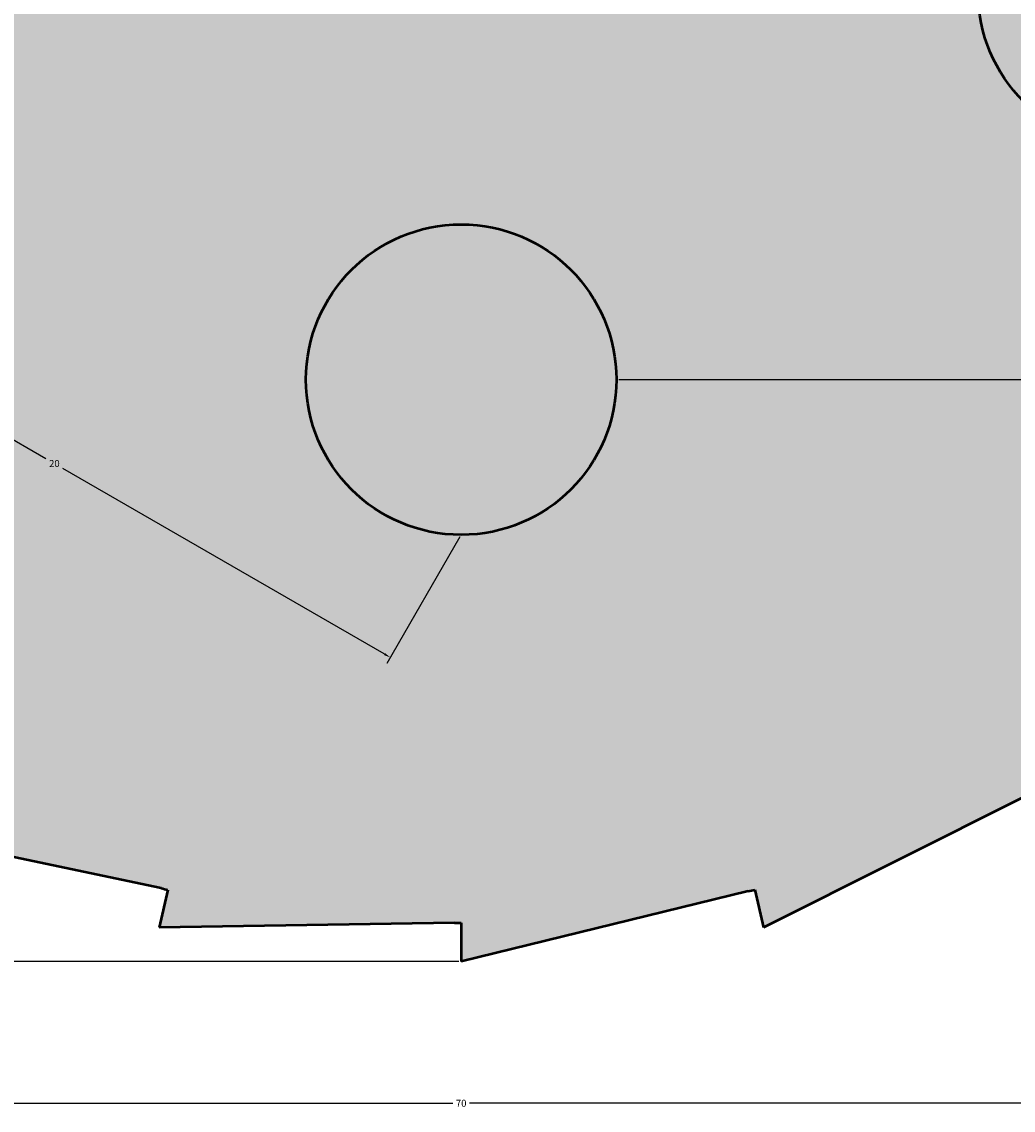
# Model space of a CAD drawing. Units: millimetres. Extents: x 2943.6 to 3032.7, y 1562 to 1639.7.
# Tile 2 of 9: x 2971.1 to 2996.7, y 1562 to 1590.1. Entities that reach past the tile are written whole.
import ezdxf

# ---------------------------------------------------------------- set-up
doc = ezdxf.new("R2010")
doc.units = ezdxf.units.MM
doc.layers.add('M-DIMS', color=2, linetype='Continuous', lineweight=18)
doc.layers.add('M-OUTL', color=7, linetype='Continuous', lineweight=50)
doc.layers.add('M-HATC', color=7, linetype='Continuous', lineweight=18, true_color=0xffffff)
doc.styles.get("Standard").update_dxf_attribs({"font": 'arial.ttf'})
doc.dimstyles.get("Standard").update_dxf_attribs({"dimtxt": 0.18, "dimasz": 0.18, "dimexe": 0.18, "dimexo": 0.0625, "dimgap": 0.09, "dimtad": 0, "dimtih": 1, "dimtoh": 1, "dimdec": 4, "dimzin": 0, "dimdsep": 46, "dimtxsty": 'Standard', "dimcen": 0.09, "dimadec": 0, "dimazin": 0, "dimtfac": 1, "dimtdec": 4, "dimtofl": 0, "dimtmove": 0, "dimatfit": 3, "dimfxl": 1, "dimtolj": 1, "dimtzin": 0, "dimarcsym": 0})

# ---------------------------------------------------------------- blocks, each defined once
blk = doc.blocks.new('*U1')
blk.add_circle((0, 0), 4)
blk = doc.blocks.new('*U2')
at = {"layer": 'M-OUTL', "color": 0, "linetype": 'ByBlock', "lineweight": -2, "transparency": 16777216}
for p, rotation in [((2999.79, 1590.848), 240), ((2982.469, 1580.848), 180)]:
    blk.add_blockref('*U1', p, dxfattribs=dict(at, rotation=rotation))
blk = doc.blocks.new('*D3')
at = {"layer": 'Defpoints', "color": 0, "transparency": 16777216}
for p in [(2947.469, 1600.848), (3017.469, 1600.848), (3017.469, 1562.198)]:
    blk.add_point(p, dxfattribs=at)
at = {"layer": 'M-DIMS', "color": 0, "lineweight": -2, "transparency": 16777216}
for p, q in [((2947.469, 1600.786), (2947.469, 1562.018)), ((3017.469, 1600.786), (3017.469, 1562.018)), ((2947.649, 1562.198), (2982.251, 1562.198)), ((3017.289, 1562.198), (2982.687, 1562.198))]:
    blk.add_line(p, q, dxfattribs=at)
at = {"layer": 'M-DIMS', "color": 0, "transparency": 16777216}
for points in [[(2947.649, 1562.228), (2947.649, 1562.168), (2947.469, 1562.198)], [(3017.289, 1562.228), (3017.289, 1562.168), (3017.469, 1562.198)]]:
    blk.add_solid(points, dxfattribs=at)
at = {"layer": 'M-DIMS', "color": 0, "transparency": 16777216, "insert": (2982.469, 1562.198), "char_height": 0.18, "attachment_point": 5}
blk.add_mtext('\\A1;70', dxfattribs=at)
blk = doc.blocks.new('*D4')
at = {"layer": 'Defpoints', "color": 0, "transparency": 16777216}
for p in [(2943.819, 1635.848), (2982.469, 1635.848), (2982.469, 1565.848)]:
    blk.add_point(p, dxfattribs=at)
at = {"layer": 'M-DIMS', "color": 0, "lineweight": -2, "transparency": 16777216}
for p, q in [((2982.407, 1635.848), (2943.639, 1635.848)), ((2943.819, 1635.668), (2943.819, 1601.03)), ((2943.819, 1566.028), (2943.819, 1600.666)), ((2982.407, 1565.848), (2943.639, 1565.848))]:
    blk.add_line(p, q, dxfattribs=at)
at = {"layer": 'M-DIMS', "color": 0, "transparency": 16777216}
for points in [[(2943.789, 1635.668), (2943.849, 1635.668), (2943.819, 1635.848)], [(2943.789, 1566.028), (2943.849, 1566.028), (2943.819, 1565.848)]]:
    blk.add_solid(points, dxfattribs=at)
at = {"layer": 'M-DIMS', "color": 0, "transparency": 16777216, "insert": (2943.819, 1600.848), "char_height": 0.18, "attachment_point": 5}
blk.add_mtext('\\A1;70', dxfattribs=at)
blk = doc.blocks.new('*D5')
at = {"layer": 'Defpoints', "color": 0, "transparency": 16777216}
for p in [(2986.469, 1620.848), (3021.119, 1620.848), (2986.469, 1580.848)]:
    blk.add_point(p, dxfattribs=at)
at = {"layer": 'M-DIMS', "color": 0, "lineweight": -2, "transparency": 16777216}
for p, q in [((2986.532, 1620.848), (3021.299, 1620.848)), ((3021.119, 1620.668), (3021.119, 1601.03)), ((3021.119, 1581.028), (3021.119, 1600.666)), ((2986.532, 1580.848), (3021.299, 1580.848))]:
    blk.add_line(p, q, dxfattribs=at)
at = {"layer": 'M-DIMS', "color": 0, "transparency": 16777216}
for points in [[(3021.089, 1620.668), (3021.149, 1620.668), (3021.119, 1620.848)], [(3021.089, 1581.028), (3021.149, 1581.028), (3021.119, 1580.848)]]:
    blk.add_solid(points, dxfattribs=at)
at = {"layer": 'M-DIMS', "color": 0, "transparency": 16777216, "insert": (3021.119, 1600.848), "char_height": 0.18, "attachment_point": 5}
blk.add_mtext('\\A1;40', dxfattribs=at)
blk = doc.blocks.new('*D6')
at = {"layer": 'Defpoints', "color": 0, "transparency": 16777216}
for p in [(2965.149, 1586.848), (2963.324, 1583.687), (2982.469, 1576.848)]:
    blk.add_point(p, dxfattribs=at)
at = {"layer": 'M-DIMS', "color": 0, "lineweight": -2, "transparency": 16777216}
for p, q in [((2965.118, 1586.794), (2963.234, 1583.531)), ((2963.48, 1583.597), (2971.764, 1578.814)), ((2980.488, 1573.777), (2972.204, 1578.56)), ((2982.438, 1576.794), (2980.554, 1573.531))]:
    blk.add_line(p, q, dxfattribs=at)
at = {"layer": 'M-DIMS', "color": 0, "transparency": 16777216}
for points in [[(2963.495, 1583.623), (2963.465, 1583.571), (2963.324, 1583.687)], [(2980.503, 1573.803), (2980.473, 1573.751), (2980.644, 1573.687)]]:
    blk.add_solid(points, dxfattribs=at)
at = {"layer": 'M-DIMS', "color": 0, "transparency": 16777216, "insert": (2971.984, 1578.687), "char_height": 0.18, "attachment_point": 5}
blk.add_mtext('\\A1;20', dxfattribs=at)

msp = doc.modelspace()

# ---------------------------------------------------------------- hatches: boundary and pattern name
at = {"layer": 'M-HATC'}
h = msp.add_hatch(color=256, dxfattribs=at)
h.set_gradient(color1=(0, 0, 255), color2=(255, 255, 0), tint=1, name='INVCURVED')
h.paths.add_polyline_path([(2949.361, 1608.583, 0.001279), (2949.322, 1608.414), (2948.347, 1608.637), (2948.473, 1600.848), (2947.469, 1600.848), (2949.283, 1593.452, 0.001279), (2949.322, 1593.283), (2948.347, 1593.06), (2951.761, 1586.253, 0.001279), (2951.836, 1586.096), (2950.935, 1585.662), (2955.779, 1579.786, 0.001279), (2955.887, 1579.65), (2955.105, 1579.026), (2961.135, 1574.375, 0.001279), (2961.271, 1574.266), (2960.647, 1573.484), (2967.561, 1570.291, 0.001279), (2967.717, 1570.215), (2967.283, 1569.314), (2974.734, 1567.74, 0.001279), (2974.904, 1567.701), (2974.681, 1566.726), (2982.295, 1566.849, 0.001279), (2982.469, 1566.848), (2982.469, 1565.848), (2989.865, 1567.662, 0.001279), (2990.035, 1567.701), (2990.258, 1566.726), (2997.064, 1570.14, 0.001279), (2997.221, 1570.215), (2997.655, 1569.314), (3003.532, 1574.158, 0.001279), (3003.668, 1574.266), (3004.291, 1573.484), (3008.943, 1579.514, 0.001279), (3009.052, 1579.65), (3009.833, 1579.026), (3013.026, 1585.94, 0.001279), (3013.102, 1586.096), (3014.003, 1585.662), (3015.578, 1593.113, 0.001279), (3015.617, 1593.283), (3016.592, 1593.06), (3016.469, 1600.674, 0.001279), (3016.469, 1600.848), (3017.469, 1600.848), (3015.655, 1608.244, 0.001279), (3015.617, 1608.414), (3016.592, 1608.637), (3013.177, 1615.443, 0.001279), (3013.102, 1615.6), (3014.003, 1616.034), (3009.16, 1621.911, 0.001279), (3009.052, 1622.047), (3009.833, 1622.67), (3003.804, 1627.322, 0.001279), (3003.668, 1627.431), (3004.291, 1628.212), (2997.378, 1631.405, 0.001279), (2997.221, 1631.481), (2997.655, 1632.382), (2990.204, 1633.957, 0.001279), (2990.035, 1633.996), (2990.258, 1634.971), (2982.469, 1634.845), (2982.469, 1635.848), (2975.073, 1634.034, 0.001279), (2974.904, 1633.996), (2974.681, 1634.971), (2967.874, 1631.556, 0.001279), (2967.717, 1631.481), (2967.283, 1632.382), (2961.407, 1627.539, 0.001279), (2961.271, 1627.431), (2960.647, 1628.212), (2955.996, 1622.183, 0.001279), (2955.887, 1622.047), (2955.105, 1622.67), (2951.912, 1615.757, 0.001279), (2951.836, 1615.6), (2950.935, 1616.034)])
h.paths.add_polyline_path([(2969.149, 1610.848, -1), (2961.149, 1610.848, -1)], flags=16)
h.paths.add_polyline_path([(2969.149, 1590.848, -1), (2961.149, 1590.848, -1)], flags=16)
h.paths.add_polyline_path([(2992.469, 1600.848, -1), (2972.469, 1600.848, -1)], flags=16)
h.paths.add_polyline_path([(2978.469, 1620.848, -1), (2986.469, 1620.848, -1)], flags=16)
h.paths.add_polyline_path([(2981.469, 1605.236), (2981.469, 1606.848), (2983.469, 1606.848), (2983.469, 1605.236, -8.887482)], flags=0)
h.paths.add_polyline_path([(2986.469, 1580.848, -1), (2978.469, 1580.848, -1)], flags=16)
h.paths.add_polyline_path([(3003.79, 1610.848, -1), (2995.79, 1610.848, -1)], flags=16)
h.paths.add_polyline_path([(3003.79, 1590.848, -1), (2995.79, 1590.848, -1)], flags=16)
h = msp.add_hatch(color=256, dxfattribs=at)
h.paths.add_polyline_path([(2978.469, 1620.848, 1), (2986.469, 1620.848, 1)])
h.paths.add_polyline_path([(2995.79, 1610.848, 1), (3003.79, 1610.848, 1)])
h.paths.add_polyline_path([(3003.79, 1590.848, 1), (2995.79, 1590.848, 1)])
h.paths.add_polyline_path([(2986.469, 1580.848, 1), (2978.469, 1580.848, 1)])
h.paths.add_polyline_path([(2969.149, 1590.848, 1), (2961.149, 1590.848, 1)])
h.paths.add_polyline_path([(2961.149, 1610.848, 1), (2969.149, 1610.848, 1)])

# ---------------------------------------------------------------- linework, layer by layer
at = {"layer": 'M-OUTL'}
for p, q in [((2997.064, 1570.14), (2990.258, 1566.726)), ((2974.734, 1567.74), (2967.283, 1569.314)), ((2974.904, 1567.701), (2974.681, 1566.726)), ((2989.865, 1567.662), (2982.469, 1565.848)), ((2990.035, 1567.701), (2990.258, 1566.726)), ((2982.295, 1566.849), (2974.681, 1566.726)), ((2982.469, 1566.848), (2982.469, 1565.848))]:
    msp.add_line(p, q, dxfattribs=at)
for start, end in [(256.8498, 257.1429), (282.564, 282.8571), (269.7069, 270)]:
    msp.add_arc((2982.469, 1600.848), 34, start, end, dxfattribs=at)

# ---------------------------------------------------------------- block references
msp.add_blockref('*U2', (0, 0), dxfattribs=at)

# ---------------------------------------------------------------- dimensions: what is measured, and where the dimension line sits
at = {"layer": 'M-DIMS'}
for base, p1, p2, angle, picture, middle in [((2943.819, 1635.848), (2982.469, 1565.848), (2982.469, 1635.848), 90, '*D4', (2943.819, 1600.848)), ((3021.119, 1620.848), (2986.469, 1580.848), (2986.469, 1620.848), 90, '*D5', (3021.119, 1600.848)), ((2963.324, 1583.687), (2982.469, 1576.848), (2965.149, 1586.848), 150, '*D6', (2971.984, 1578.687))]:
    dim = msp.add_linear_dim(base=base, p1=p1, p2=p2, angle=angle, dimstyle='Standard', override={"dimdec": 0, "dimlfac": 1, "dimrnd": 0, "dimzin": 0, "dimdsep": 46, "dimlunit": 2}, dxfattribs=at)
    dim.commit()
    dim.dimension.update_dxf_attribs({"geometry": picture, "text_midpoint": middle})
dim = msp.add_linear_dim(base=(3017.469, 1562.198), p1=(2947.469, 1600.848), p2=(3017.469, 1600.848), dimstyle='Standard', override={"dimdec": 0, "dimlfac": 1, "dimrnd": 0, "dimzin": 0, "dimdsep": 46, "dimlunit": 2}, dxfattribs=at)
dim.commit()
dim.dimension.update_dxf_attribs({"geometry": '*D3', "text_midpoint": (2982.469, 1562.198)})

doc.saveas('drawing.dxf')
